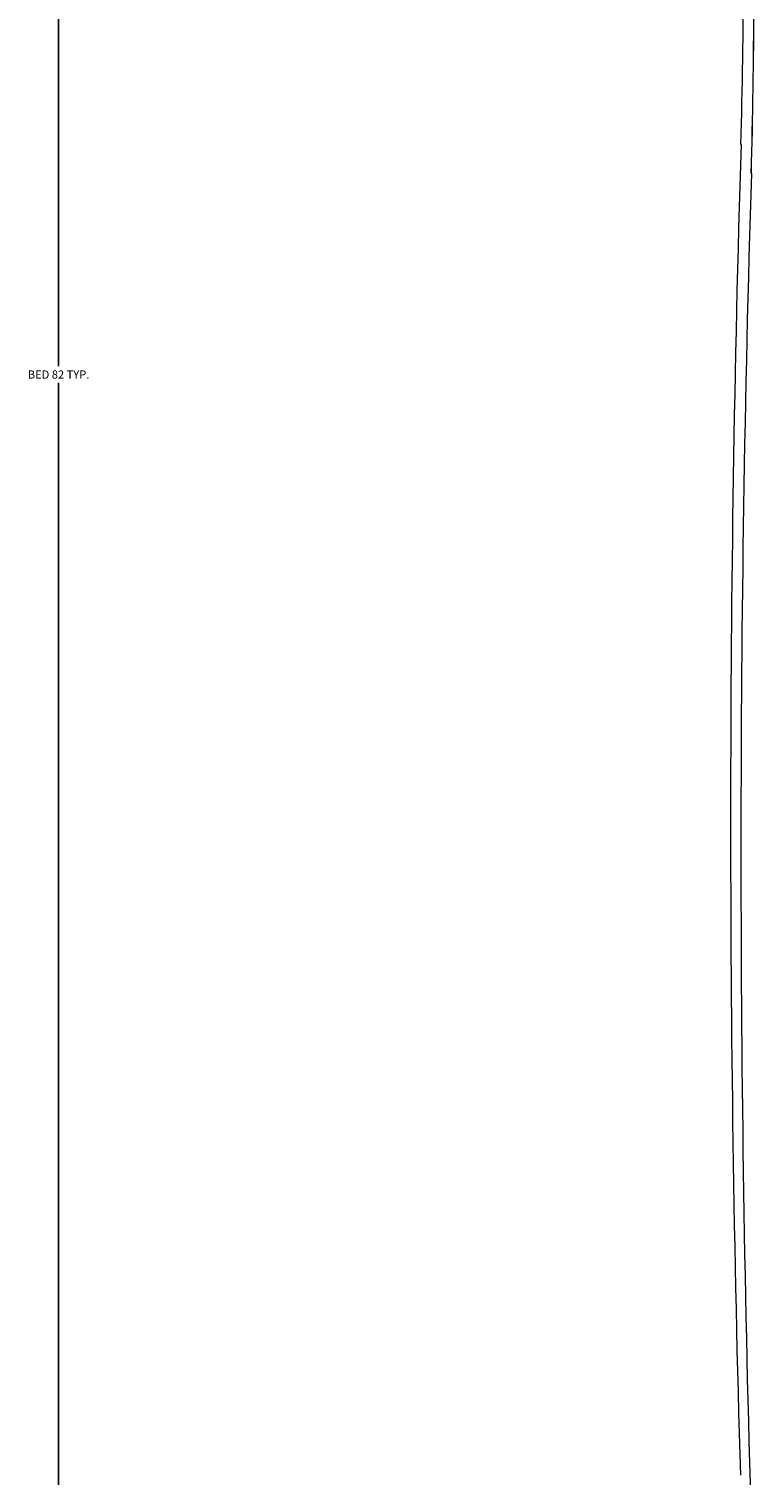
# Model space of a CAD drawing. Units: inches. Extents: x 1885 to 2748, y 783 to 2421.
# Tile 94 of 117: x 2372 to 2388, y 2282 to 2314. Entities that reach past the tile are written whole.
import ezdxf

# ---------------------------------------------------------------- set-up
doc = ezdxf.new("R2010")
doc.units = ezdxf.units.IN
doc.layers.add('A-ANNO-DIMS', color=2, linetype='Continuous', lineweight=18)
doc.layers.add('A-FURN', color=8, linetype='Continuous', lineweight=13)
doc.styles.get("Standard").update_dxf_attribs({"font": 'arial.ttf'})
doc.dimstyles.get("Standard").update_dxf_attribs({"dimtxt": 0.18, "dimasz": 0.18, "dimexe": 0.18, "dimexo": 0.0625, "dimgap": 0.09, "dimtad": 0, "dimtih": 1, "dimtoh": 1, "dimdec": 4, "dimzin": 0, "dimdsep": 46, "dimtxsty": 'Standard', "dimcen": 0.09, "dimadec": 0, "dimazin": 0, "dimtfac": 1, "dimtdec": 4, "dimtofl": 0, "dimtmove": 0, "dimatfit": 3, "dimfxl": 1, "dimtolj": 1, "dimtzin": 0, "dimarcsym": 0})

# ---------------------------------------------------------------- blocks, each defined once
blk = doc.blocks.new('BED-DOUBLE')
for centre, radius, start, end in [((31.817, -167.08), 170.11, 88.4762, 91.00819), ((31.817, -167.081), 170.11, 88.4762, 91.00819), ((51.257, 485.049), 482.31, 268.22771, 271.71854), ((51.257, 485.049), 482.31, 268.22771, 271.71854), ((31.177, -167.309), 170.11, 88.4762, 91.00819), ((31.177, -167.309), 170.11, 88.4762, 91.00819), ((50.617, 484.821), 482.31, 268.22771, 271.71854), ((50.617, 484.821), 482.31, 268.22771, 271.71854)]:
    blk.add_arc(centre, radius, start, end)
blk = doc.blocks.new('*D27')
at = {"layer": 'A-ANNO-DIMS', "color": 0, "lineweight": -2, "transparency": 16777216}
for p, q in [((2385.079, 2346.649), (2372.729, 2346.649)), ((2372.909, 2346.469), (2372.909, 2306.056)), ((2372.909, 2265.28), (2372.909, 2305.693)), ((2385.079, 2265.1), (2372.729, 2265.1))]:
    blk.add_line(p, q, dxfattribs=at)
at = {"layer": 'A-ANNO-DIMS', "color": 0, "transparency": 16777216}
for points in [[(2372.879, 2346.469), (2372.939, 2346.469), (2372.909, 2346.649)], [(2372.879, 2265.28), (2372.939, 2265.28), (2372.909, 2265.1)]]:
    blk.add_solid(points, dxfattribs=at)
at = {"layer": 'Defpoints', "color": 0, "transparency": 16777216}
for p in [(2385.141, 2346.649), (2372.909, 2265.1), (2385.141, 2265.1)]:
    blk.add_point(p, dxfattribs=at)
at = {"layer": 'A-ANNO-DIMS', "color": 0, "transparency": 16777216, "insert": (2372.909, 2305.874), "char_height": 0.18, "attachment_point": 5}
blk.add_mtext('\\A1;BED 82 TYP.', dxfattribs=at)

msp = doc.modelspace()

# ---------------------------------------------------------------- block references
at = {"layer": 'A-FURN', "rotation": 269.9999998331857}
msp.add_blockref('BED-DOUBLE', (2385.229, 2346.652), dxfattribs=at)

# ---------------------------------------------------------------- dimensions: what is measured, and where the dimension line sits
at = {"layer": 'A-ANNO-DIMS'}
dim = msp.add_linear_dim(base=(2372.909, 2265.1), p1=(2385.141, 2346.649), p2=(2385.141, 2265.1), angle=270, text='BED <> TYP.', dimstyle='Standard', override={"dimdec": 0, "dimlfac": 1, "dimrnd": 0, "dimzin": 0, "dimdsep": 46, "dimlunit": 2}, dxfattribs=at)
dim.commit()
dim.dimension.update_dxf_attribs({"geometry": '*D27', "text_midpoint": (2372.909, 2305.874)})

doc.saveas('drawing.dxf')
